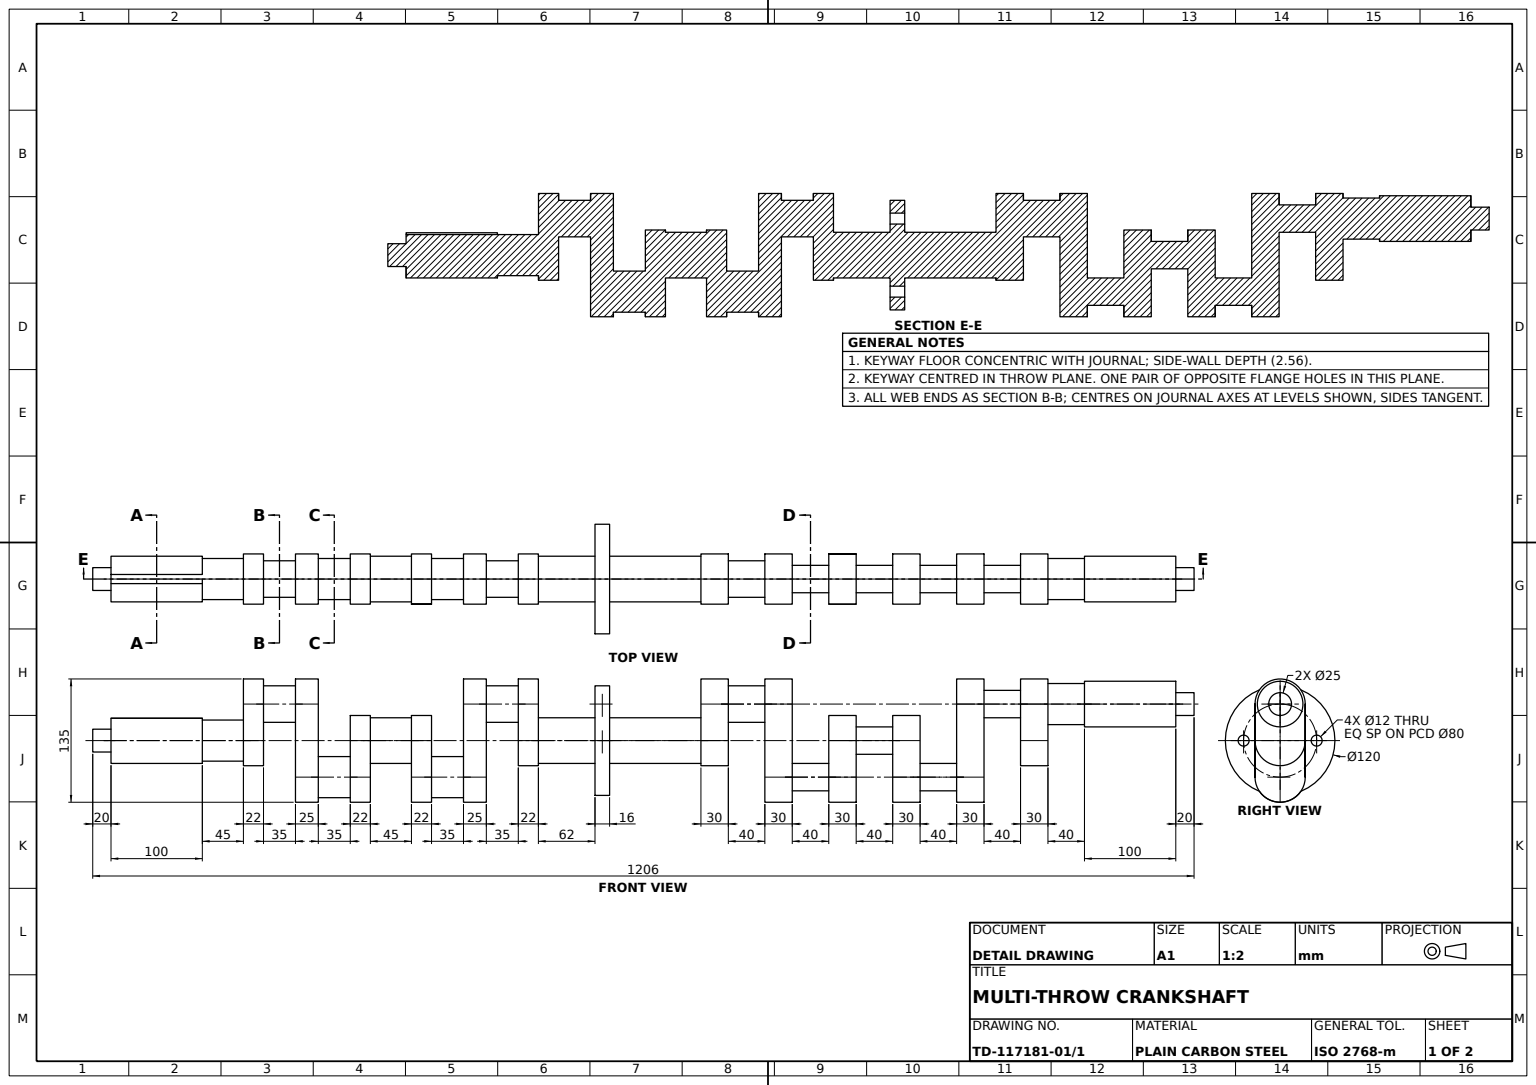
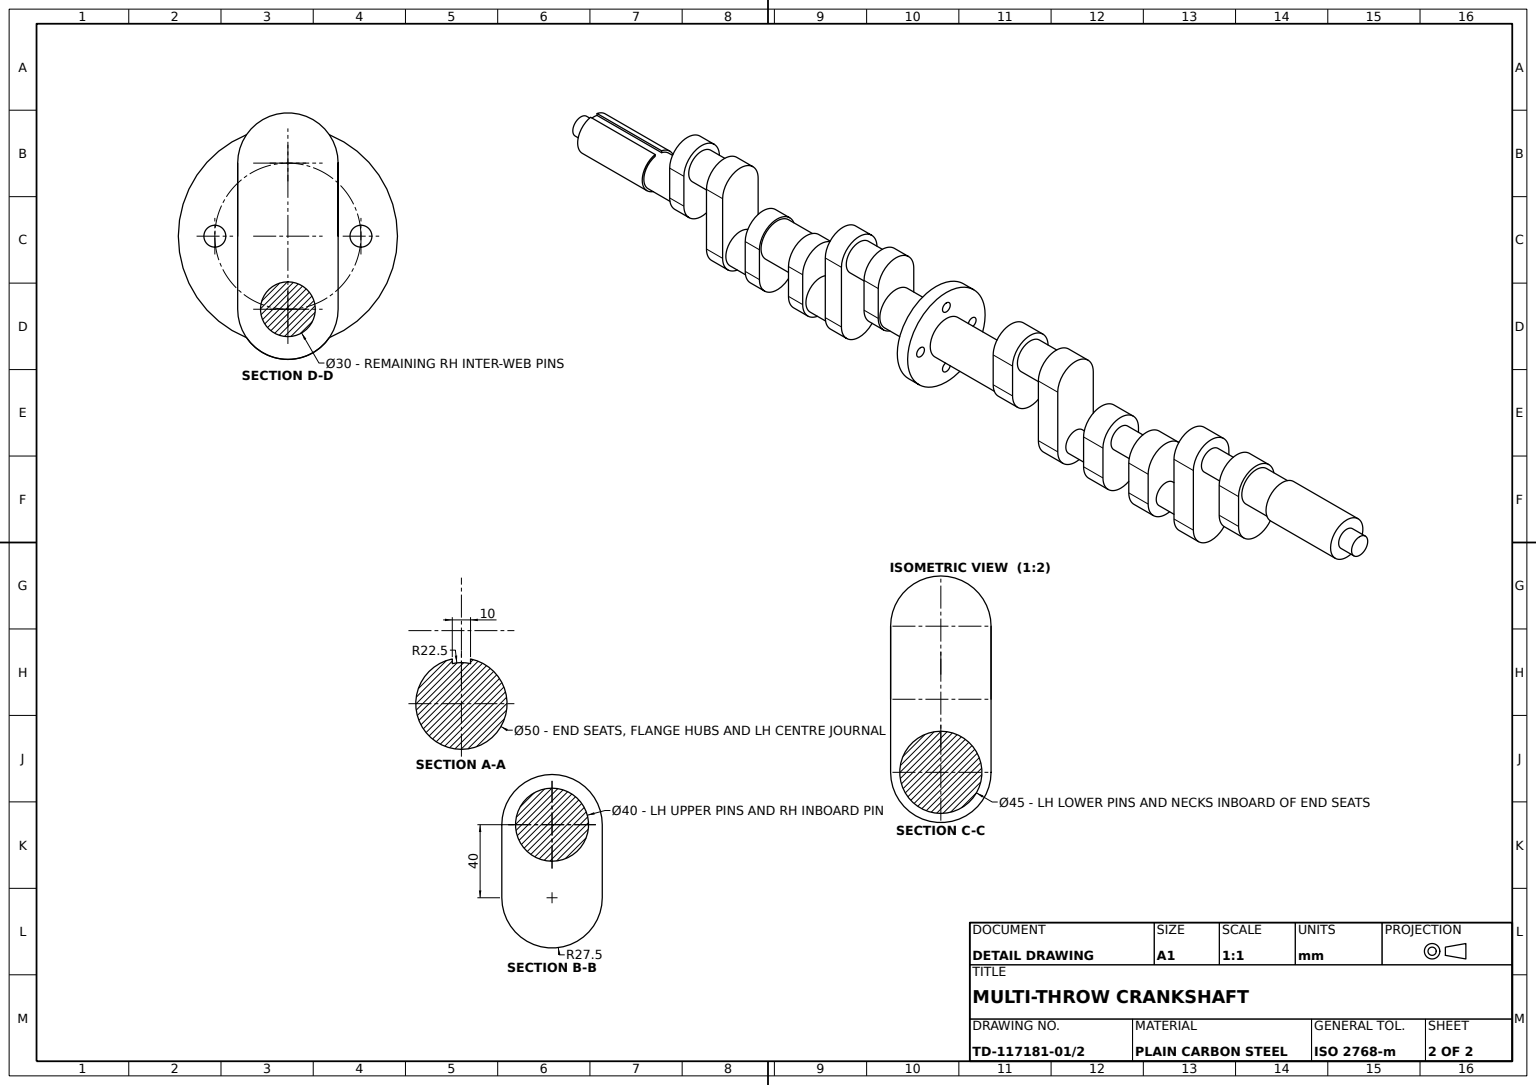
from build123d import *

# Parameters (mm, degrees)
CENTRE_FLANGE_SKETCH_R  = 60
CENTRE_FLANGE_120_DEPTH = 16
FLANGE_HOLES_SKETCH_R   = 6
FLANGE_HOLES_12_DEPTH   = 87.34813258
A_JOURNAL_1_SKETCH_R    = 25
A_JOURNAL_1_50_DEPTH    = 62
A_WEB_1_DEPTH           = 22
A_PIN_1_SKETCH_R        = 20
A_PIN_1_40_DEPTH        = 35
A_WEB_2_DEPTH           = 25
A_PIN_2_SKETCH_R        = 22.5
A_PIN_2_45_DEPTH        = 35
A_WEB_3_DEPTH           = 22
A_JOURNAL_2_SKETCH_R    = 25
A_JOURNAL_2_50_DEPTH    = 45
A_WEB_4_DEPTH           = 22
A_PIN_3_SKETCH_R        = 22.5
A_PIN_3_45_DEPTH        = 35
A_WEB_5_DEPTH           = 25
A_PIN_4_SKETCH_R        = 20
A_PIN_4_40_DEPTH        = 35
A_WEB_6_DEPTH           = 22
A_JOURNAL_3_SKETCH_R    = 22.5
A_JOURNAL_3_45_DEPTH    = 45
A_SHAFT_END_DEPTH       = 100
A_END_SPIGOT_SKETCH_R   = 12.5
A_END_SPIGOT_25_DEPTH   = 20
B_START                 = 100
B_JOURNAL_1_SKETCH_R    = 25
B_JOURNAL_1_50_DEPTH    = 100
B_START_2               = 30
B_WEB_1_DEPTH           = 30
B_START_3               = 40
B_PIN_1_SKETCH_R        = 20
B_PIN_1_40_DEPTH        = 40
B_WEB_2_DEPTH           = 30
B_JOURNAL_2_SKETCH_R    = 15
B_JOURNAL_2_30_DEPTH    = 40
B_WEB_3_DEPTH           = 30
B_JOURNAL_3_SKETCH_R    = 15
B_JOURNAL_3_30_DEPTH    = 40
B_WEB_4_DEPTH           = 30
B_JOURNAL_4_SKETCH_R    = 15
B_JOURNAL_4_30_DEPTH    = 40
B_WEB_5_DEPTH           = 30
B_JOURNAL_5_SKETCH_R    = 15
B_JOURNAL_5_30_DEPTH    = 40
B_WEB_6_DEPTH           = 30
B_JOURNAL_6_SKETCH_R    = 22.5
B_JOURNAL_6_45_DEPTH    = 40
B_SHAFT_END_SKETCH_R    = 25
B_SHAFT_END_50_DEPTH    = 100
B_END_SPIGOT_SKETCH_R   = 12.5
B_END_SPIGOT_25_DEPTH   = 20


with BuildPart() as part:
    # Centre Flange Sketch → Centre Flange Ø120 (new body)
    with BuildSketch(Plane.XY):
        Circle(CENTRE_FLANGE_SKETCH_R)
    extrude(amount=CENTRE_FLANGE_120_DEPTH)

    # Flange Holes Sketch → Flange Holes Ø12 (cut, through all)
    with BuildSketch(Plane.XY.offset(16)):
        with Locations((0, 40)):
            Circle(FLANGE_HOLES_SKETCH_R)
        with Locations((40, 0)):
            Circle(FLANGE_HOLES_SKETCH_R)
        with Locations((0, -40)):
            Circle(FLANGE_HOLES_SKETCH_R)
        with Locations((-40, 0)):
            Circle(FLANGE_HOLES_SKETCH_R)
    extrude(amount=-FLANGE_HOLES_12_DEPTH, mode=Mode.SUBTRACT)

    # A Journal 1 Sketch → A Journal 1 Ø50 (add)
    with BuildSketch(Plane.XY.offset(16)):
        Circle(A_JOURNAL_1_SKETCH_R)
    extrude(amount=A_JOURNAL_1_50_DEPTH)

    # A Web 1 Sketch → A Web 1 (add)
    with BuildSketch(Plane.XY.offset(78)):
        with BuildLine():
            Line((0, -27.5), (-40, -27.5))
            ThreePointArc((-40, -27.5), (-67.5, 0), (-40, 27.5))
            Line((-40, 27.5), (0, 27.5))
            ThreePointArc((0, 27.5), (27.5, 0), (0, -27.5))
        make_face()
    extrude(amount=A_WEB_1_DEPTH)

    # A Pin 1 Sketch → A Pin 1 Ø40 (add)
    with BuildSketch(Plane.XY.offset(100)):
        with Locations((-40, 0)):
            Circle(A_PIN_1_SKETCH_R)
    extrude(amount=A_PIN_1_40_DEPTH)

    # A Web 2 Sketch → A Web 2 (add)
    with BuildSketch(Plane.XY.offset(135)):
        with BuildLine():
            Line((-40, 27.5), (40, 27.5))
            ThreePointArc((40, 27.5), (67.5, 0), (40, -27.5))
            Line((40, -27.5), (-40, -27.5))
            ThreePointArc((-40, -27.5), (-67.5, 0), (-40, 27.5))
        make_face()
    extrude(amount=A_WEB_2_DEPTH)

    # A Pin 2 Sketch → A Pin 2 Ø45 (add)
    with BuildSketch(Plane.XY.offset(160)):
        with Locations((40, 0)):
            Circle(A_PIN_2_SKETCH_R)
    extrude(amount=A_PIN_2_45_DEPTH)

    # A Web 3 Sketch → A Web 3 (add)
    with BuildSketch(Plane.XY.offset(195)):
        with BuildLine():
            Line((40, -27.5), (0, -27.5))
            ThreePointArc((0, -27.5), (-27.5, 0), (0, 27.5))
            Line((0, 27.5), (40, 27.5))
            ThreePointArc((40, 27.5), (67.5, 0), (40, -27.5))
        make_face()
    extrude(amount=A_WEB_3_DEPTH)

    # A Journal 2 Sketch → A Journal 2 Ø50 (add)
    with BuildSketch(Plane.XY.offset(217)):
        Circle(A_JOURNAL_2_SKETCH_R)
    extrude(amount=A_JOURNAL_2_50_DEPTH)

    # A Web 4 Sketch → A Web 4 (add)
    with BuildSketch(Plane.XY.offset(262)):
        with BuildLine():
            Line((0, 27.5), (40, 27.5))
            ThreePointArc((40, 27.5), (67.5, 0), (40, -27.5))
            Line((40, -27.5), (0, -27.5))
            ThreePointArc((0, -27.5), (-27.5, 0), (0, 27.5))
        make_face()
    extrude(amount=A_WEB_4_DEPTH)

    # A Pin 3 Sketch → A Pin 3 Ø45 (add)
    with BuildSketch(Plane.XY.offset(284)):
        with Locations((40, 0)):
            Circle(A_PIN_3_SKETCH_R)
    extrude(amount=A_PIN_3_45_DEPTH)

    # A Web 5 Sketch → A Web 5 (add)
    with BuildSketch(Plane.XY.offset(319)):
        with BuildLine():
            Line((40, -27.5), (-40, -27.5))
            ThreePointArc((-40, -27.5), (-67.5, 0), (-40, 27.5))
            Line((-40, 27.5), (40, 27.5))
            ThreePointArc((40, 27.5), (67.5, 0), (40, -27.5))
        make_face()
    extrude(amount=A_WEB_5_DEPTH)

    # A Pin 4 Sketch → A Pin 4 Ø40 (add)
    with BuildSketch(Plane.XY.offset(344)):
        with Locations((-40, 0)):
            Circle(A_PIN_4_SKETCH_R)
    extrude(amount=A_PIN_4_40_DEPTH)

    # A Web 6 Sketch → A Web 6 (add)
    with BuildSketch(Plane.XY.offset(379)):
        with BuildLine():
            Line((-40, 27.5), (0, 27.5))
            ThreePointArc((0, 27.5), (27.5, 0), (0, -27.5))
            Line((0, -27.5), (-40, -27.5))
            ThreePointArc((-40, -27.5), (-67.5, 0), (-40, 27.5))
        make_face()
    extrude(amount=A_WEB_6_DEPTH)

    # A Journal 3 Sketch → A Journal 3 Ø45 (add)
    with BuildSketch(Plane.XY.offset(401)):
        with Locations(Location((0, 0, 0), (0, 0, 180))):
            Circle(A_JOURNAL_3_SKETCH_R)
    extrude(amount=A_JOURNAL_3_45_DEPTH)

    # A Shaft End Sketch → A Shaft End (add)
    with BuildSketch(Plane.XY.offset(446)):
        with BuildLine():
            Line((-24.494897428, 5), (-21.937410968, 5))
            ThreePointArc((-21.937410968, 5), (-22.5, 0), (-21.937410968, -5))
            Line((-21.937410968, -5), (-24.494897428, -5))
            ThreePointArc((-24.494897428, -5), (25, 0), (-24.494897428, 5))
        make_face()
    extrude(amount=A_SHAFT_END_DEPTH)

    # A End Spigot Sketch → A End Spigot Ø25 (add)
    with BuildSketch(Plane.XY.offset(546)):
        Circle(A_END_SPIGOT_SKETCH_R)
    extrude(amount=A_END_SPIGOT_25_DEPTH)

    # B Journal 1 Sketch → B Journal 1 Ø50 (add)
    with BuildSketch(Plane(origin=(0, 0, 0), x_dir=(-1, 0, 0), z_dir=(0, 0, -1)).offset(B_START)):
        with Locations(Location((0, 0, 0), (0, 0, 180))):
            Circle(B_JOURNAL_1_SKETCH_R)
    extrude(amount=-B_JOURNAL_1_50_DEPTH)

    # B Web 1 Sketch → B Web 1 (add)
    with BuildSketch(Plane(origin=(0, 0, -100), x_dir=(-1, 0, 0), z_dir=(0, 0, -1)).offset(B_START_2)):
        with BuildLine():
            Line((0, 27.5), (40, 27.5))
            ThreePointArc((40, 27.5), (67.5, 0), (40, -27.5))
            Line((40, -27.5), (0, -27.5))
            ThreePointArc((0, -27.5), (-27.5, 0), (0, 27.5))
        make_face()
    extrude(amount=-B_WEB_1_DEPTH)

    # B Pin 1 Sketch → B Pin 1 Ø40 (add)
    with BuildSketch(Plane(origin=(0, 0, -130), x_dir=(-1, 0, 0), z_dir=(0, 0, -1)).offset(B_START_3)):
        with Locations(Location((40, 0, 0), (0, 0, 180))):
            Circle(B_PIN_1_SKETCH_R)
    extrude(amount=-B_PIN_1_40_DEPTH)

    # B Web 2 Sketch → B Web 2 (add)
    with BuildSketch(Plane(origin=(0, 0, -170), x_dir=(-1, 0, 0), z_dir=(0, 0, -1)).offset(B_START_2)):
        with BuildLine():
            Line((40, -27.5), (-40, -27.5))
            ThreePointArc((-40, -27.5), (-67.5, 0), (-40, 27.5))
            Line((-40, 27.5), (40, 27.5))
            ThreePointArc((40, 27.5), (67.5, 0), (40, -27.5))
        make_face()
    extrude(amount=-B_WEB_2_DEPTH)

    # B Journal 2 Sketch → B Journal 2 Ø30 (add)
    with BuildSketch(Plane(origin=(0, 0, -200), x_dir=(-1, 0, 0), z_dir=(0, 0, -1))):
        with Locations((-40, 0)):
            Circle(B_JOURNAL_2_SKETCH_R)
    extrude(amount=B_JOURNAL_2_30_DEPTH)

    # B Web 3 Sketch → B Web 3 (add)
    with BuildSketch(Plane(origin=(0, 0, -240), x_dir=(-1, 0, 0), z_dir=(0, 0, -1)).offset(B_START_2)):
        with BuildLine():
            Line((-40, 27.5), (0, 27.5))
            ThreePointArc((0, 27.5), (27.5, 0), (0, -27.5))
            Line((0, -27.5), (-40, -27.5))
            ThreePointArc((-40, -27.5), (-67.5, 0), (-40, 27.5))
        make_face()
    extrude(amount=-B_WEB_3_DEPTH)

    # B Journal 3 Sketch → B Journal 3 Ø30 (add)
    with BuildSketch(Plane(origin=(0, 0, -270), x_dir=(-1, 0, 0), z_dir=(0, 0, -1))):
        Circle(B_JOURNAL_3_SKETCH_R)
    extrude(amount=B_JOURNAL_3_30_DEPTH)

    # B Web 4 Sketch → B Web 4 (add)
    with BuildSketch(Plane(origin=(0, 0, -310), x_dir=(-1, 0, 0), z_dir=(0, 0, -1)).offset(B_START_2)):
        with BuildLine():
            Line((0, -27.5), (-40, -27.5))
            ThreePointArc((-40, -27.5), (-67.5, 0), (-40, 27.5))
            Line((-40, 27.5), (0, 27.5))
            ThreePointArc((0, 27.5), (27.5, 0), (0, -27.5))
        make_face()
    extrude(amount=-B_WEB_4_DEPTH)

    # B Journal 4 Sketch → B Journal 4 Ø30 (add)
    with BuildSketch(Plane(origin=(0, 0, -340), x_dir=(-1, 0, 0), z_dir=(0, 0, -1))):
        with Locations((-40, 0)):
            Circle(B_JOURNAL_4_SKETCH_R)
    extrude(amount=B_JOURNAL_4_30_DEPTH)

    # B Web 5 Sketch → B Web 5 (add)
    with BuildSketch(Plane(origin=(0, 0, -380), x_dir=(-1, 0, 0), z_dir=(0, 0, -1)).offset(B_START_2)):
        with BuildLine():
            Line((-40, 27.5), (40, 27.5))
            ThreePointArc((40, 27.5), (67.5, 0), (40, -27.5))
            Line((40, -27.5), (-40, -27.5))
            ThreePointArc((-40, -27.5), (-67.5, 0), (-40, 27.5))
        make_face()
    extrude(amount=-B_WEB_5_DEPTH)

    # B Journal 5 Sketch → B Journal 5 Ø30 (add)
    with BuildSketch(Plane(origin=(0, 0, -410), x_dir=(-1, 0, 0), z_dir=(0, 0, -1))):
        with Locations((40, 0)):
            Circle(B_JOURNAL_5_SKETCH_R)
    extrude(amount=B_JOURNAL_5_30_DEPTH)

    # B Web 6 Sketch → B Web 6 (add)
    with BuildSketch(Plane(origin=(0, 0, -450), x_dir=(-1, 0, 0), z_dir=(0, 0, -1)).offset(B_START_2)):
        with BuildLine():
            Line((40, -27.5), (0, -27.5))
            ThreePointArc((0, -27.5), (-27.5, 0), (0, 27.5))
            Line((0, 27.5), (40, 27.5))
            ThreePointArc((40, 27.5), (67.5, 0), (40, -27.5))
        make_face()
    extrude(amount=-B_WEB_6_DEPTH)

    # B Journal 6 Sketch → B Journal 6 Ø45 (add)
    with BuildSketch(Plane(origin=(0, 0, -480), x_dir=(-1, 0, 0), z_dir=(0, 0, -1))):
        with Locations((40, 0)):
            Circle(B_JOURNAL_6_SKETCH_R)
    extrude(amount=B_JOURNAL_6_45_DEPTH)

    # B Shaft End Sketch → B Shaft End Ø50 (add)
    with BuildSketch(Plane(origin=(0, 0, -520), x_dir=(-1, 0, 0), z_dir=(0, 0, -1))):
        with Locations((40, 0)):
            Circle(B_SHAFT_END_SKETCH_R)
    extrude(amount=B_SHAFT_END_50_DEPTH)

    # B End Spigot Sketch → B End Spigot Ø25 (add)
    with BuildSketch(Plane(origin=(0, 0, -620), x_dir=(-1, 0, 0), z_dir=(0, 0, -1))):
        with Locations((40, 0)):
            Circle(B_END_SPIGOT_SKETCH_R)
    extrude(amount=B_END_SPIGOT_25_DEPTH)


solid = part.part
